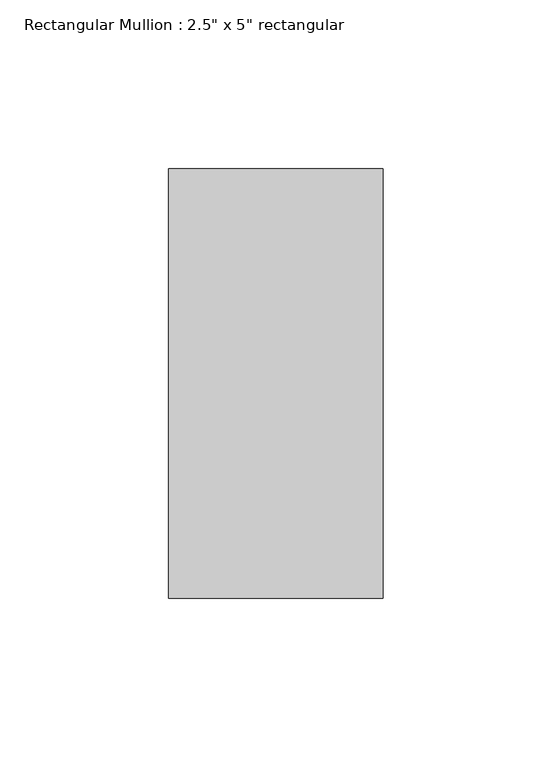
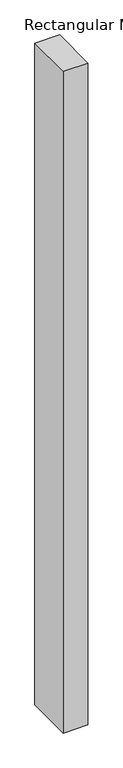
"""IFC4 building model written with IfcOpenShell, lengths in millimetres: member geometry."""

from ifc_helpers import new_model, si_unit, frame, origin, place, context, project, spatial, polyline, outline, extrude, source, transform, mapped, element, save


def member_f67b4128(model_context):
    return source(origin(), model_context, "Body", "SweptSolid", [
        extrude(outline(polyline([(0.0, 63.5), (0.0, -63.5), (-63.5, -63.5), (-63.5, 63.5), (0.0, 63.5)])), frame((0.0, 0.0, -1805.4265918), z_axis=(0.0, 0.0, 1.0), x_axis=(1.0, 0.0, 0.0)), (0.0, 0.0, 1.0), 1805.4265918),
    ])


if __name__ == "__main__":
    model = new_model("IFC4")
    model_context = context("Model", 3, world=origin())
    ifc_project = project(units=[si_unit("LENGTHUNIT", "METRE", prefix="MILLI")], contexts=[model_context])
    site = spatial("IfcSite", under=ifc_project)
    building = spatial("IfcBuilding", under=site)
    placement = place(None, origin())
    member_shape = member_f67b4128(model_context)
    element("IfcMember", 1, ObjectType="Rectangular Mullion : 2.5\" x 5\" rectangular", at=placement, inside=building, context=model_context, shape_type="MappedRepresentation", body=[
        mapped(member_shape, transform((0.0, 0.0, 0.0), x_axis=(1.0, 0.0, 0.0), y_axis=(0.0, 1.0, 0.0), z_axis=(0.0, 0.0, 1.0))),
    ])
    save(model, "model.ifc")

# Revit data of these elements
# Type "Rectangular Mullion : 2.5\" x 5\" rectangular"
#   built-in parameter 1007304 = 0.416667 (stored number, unit not read)
#   built-in parameter 1007301 = 0.104167 (stored number, unit not read)
#   built-in parameter 1007300 = 0.104167 (stored number, unit not read)
# Element 1 (IfcMember, "Rectangular Mullion : 2.5\" x 5\" rectangular")
#   Materials on its faces: "Aluminum"
# Materials
#   "Aluminum": class "Metal", colour RGB 247 247 247, transparency 0, Description = "Aluminum 6061", Cost = 0
